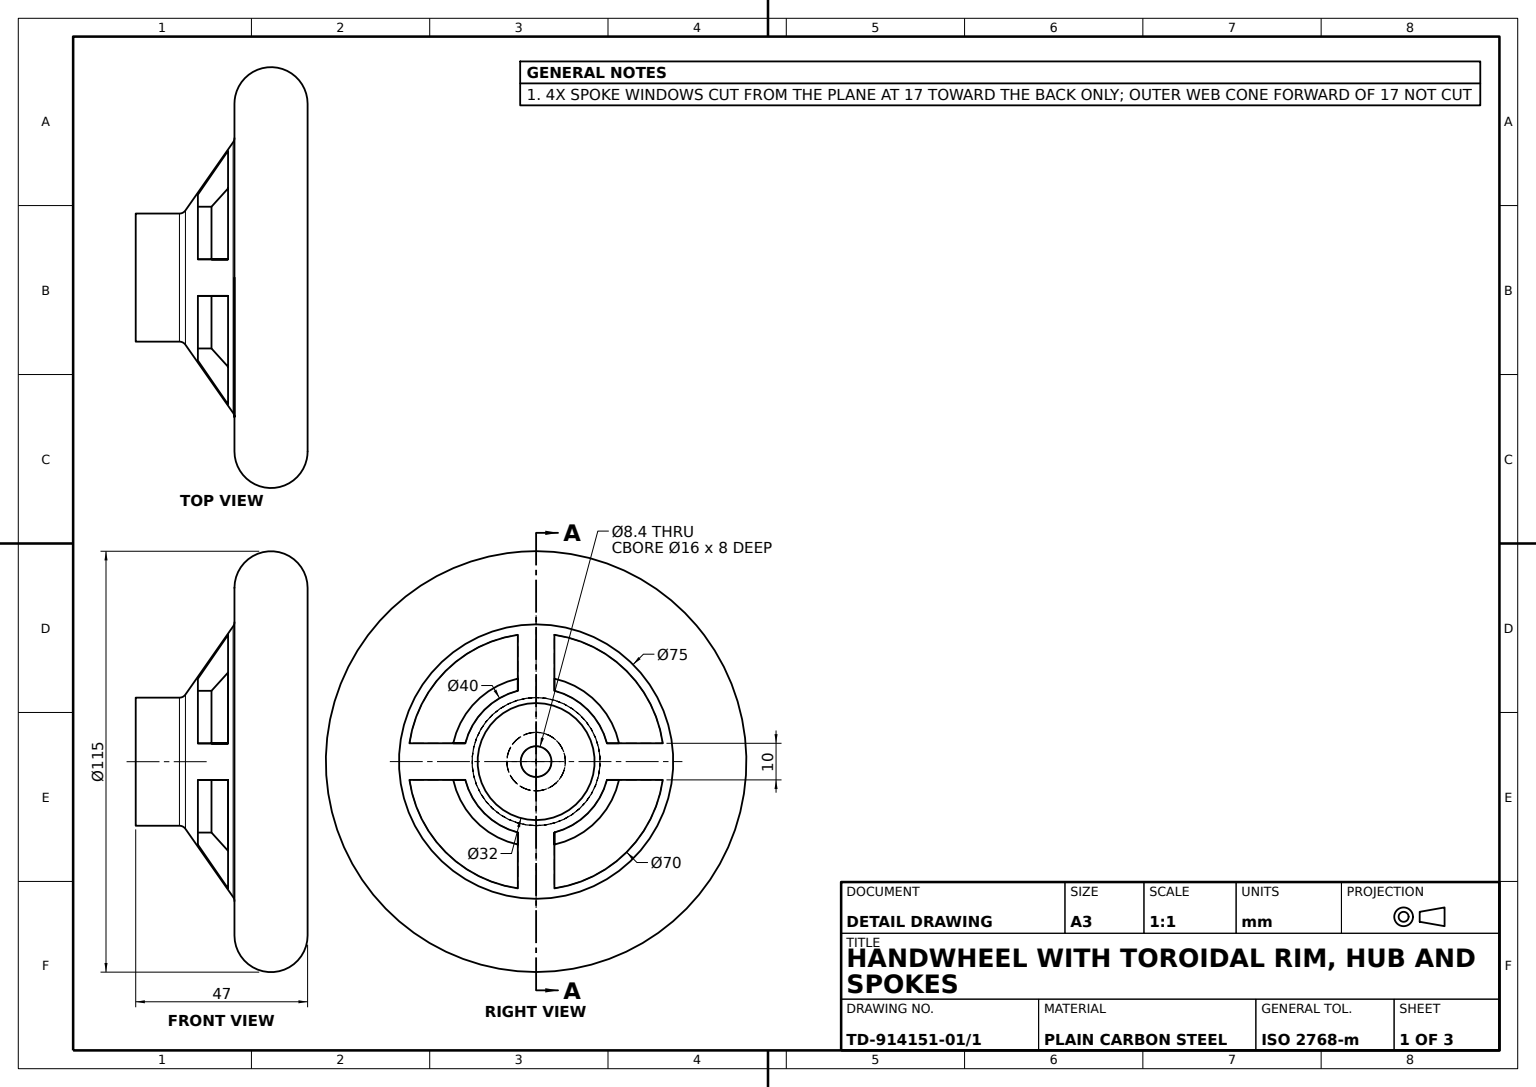
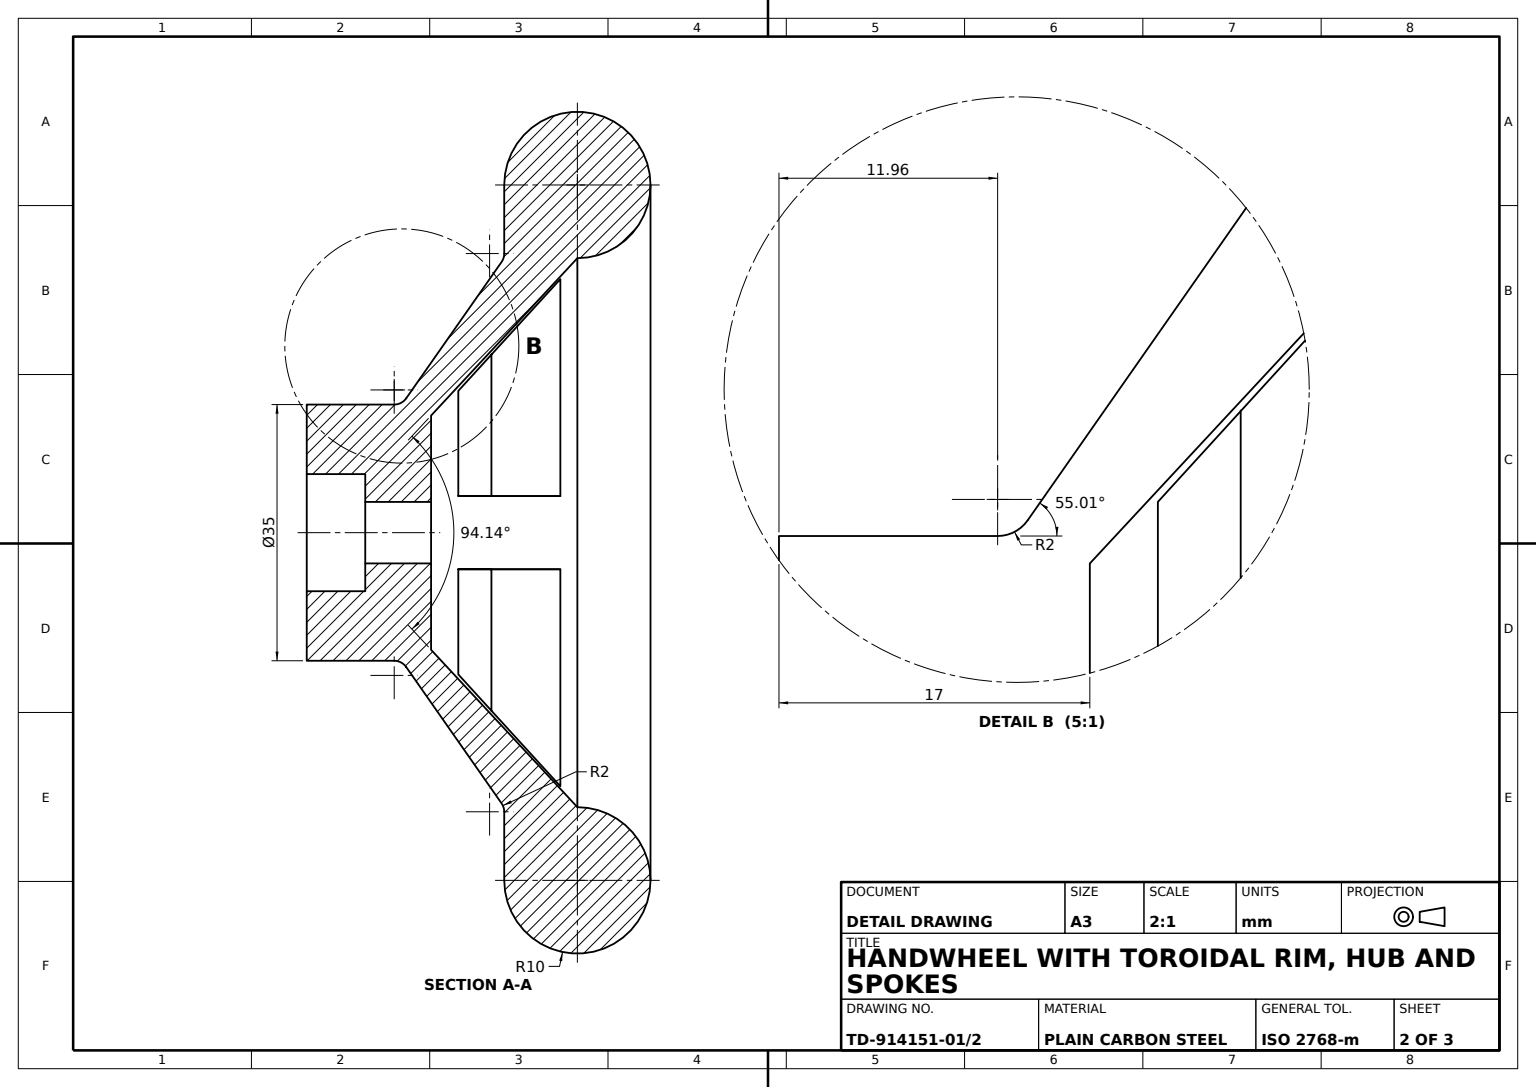
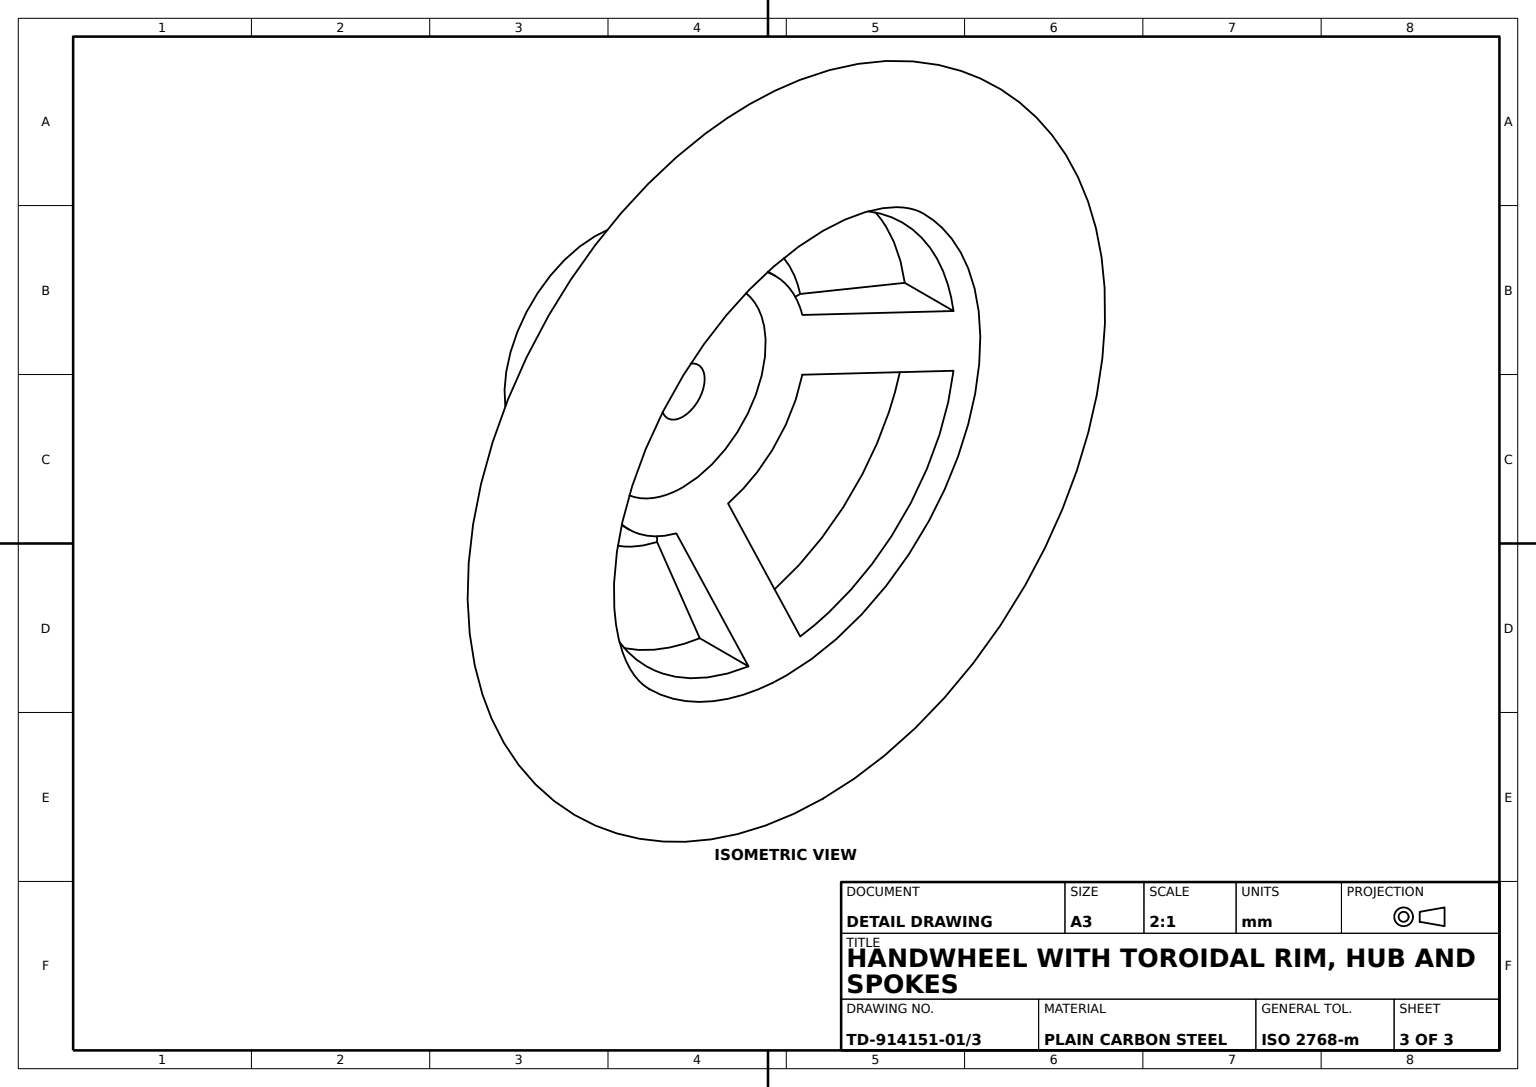
SolidWorks part; units mm, degrees
material "Plain Carbon Steel"
ref_plane "Front Plane" through (0, 0, 0) normal (0, 0, 1) x (1, 0, 0)
ref_plane "Top Plane" through (0, 0, 0) normal (0, 1, 0) x (1, 0, 0)
ref_plane "Right Plane" through (0, 0, 0) normal (1, 0, 0) x (0, 0, -1)
sketch "Handwheel Profile Sketch" plane through (0, 0, 0) normal (0, 0, 1) x (1, 0, 0)
  line L0 (0, 48.5307) -> (0, -37) construction
  line L1 (-8, -37) -> (-17.5, -37)
  line L2 (-17.5, -37) -> (-17.5, -25.0413)
  line L3 (-4.2, -20) -> (-4.2, -29)
  line L4 (-47.5, -10) -> (-38.1304, -10)
  line L5 (-36.9835, -10.3615) -> (-18.3531, -23.4028)
  line L6 (-4.2, -20) -> (-16, -20)
  line L7 (-37.5, 0) -> (-16, -20)
  line L11 (-4.2, -29) -> (-8, -29)
  line L12 (-8, -37) -> (-8, -29)
  arc A4 (-37.5, 0) -> (-47.5, -10) centre (-47.5, 0) ccw
  arc A5 (-38.1304, -10) -> (-36.9835, -10.3615) centre (-38.1304, -12) cw
  arc A6 (-17.5, -25.0413) -> (-18.3531, -23.4028) centre (-19.5, -25.0413) ccw
  point P9 (-47.5, 10)
  point P11 (0, -20)
  point P12 (-17.5, -20)
  point P16 (-37.5, -10)
  point P19 (-17.5, -24)
  point P20 (0, -37.605)
  dimension "D1" = 20
  dimension "D2" = 47.5
  dimension "D3" = 17.5
  dimension "D7" = 2
  dimension "D4" = 13
  dimension "D5" = 10
  dimension "D6" = 37
  dimension "D8" = 8
  dimension "D9" = 8
  dimension "D10" = 4.2
  dimension "D11" = 16
  dimension "D12" = 17
  dimension "D13" = 0.605
revolve "Handwheel Body" add sketch "Handwheel Profile Sketch" angle 360 about L0
sketch "Spoke Windows Sketch" plane through (0, -20, 0) normal (0, 1, 0) x (1, 0, 0)
  line L0 (0, 37.5) -> (0, -37.5) construction
  line L1 (-5, 34.641) -> (-5, 19.3649)
  line L2 (5, 34.641) -> (5, 19.3649)
  line L3 (-37.5, 0) -> (37.5, 0) construction
  line L4 (-34.641, -5) -> (-19.3649, -5)
  line L5 (-34.641, 5) -> (-19.3649, 5)
  line L6 (-5, 5) -> (-5, -5)
  line L7 (-5, 5) -> (5, 5)
  line L8 (-5, 37.5) -> (-5, -37.5) construction
  line L9 (5, 5) -> (5, -5)
  line L10 (-37.5, 5) -> (37.5, 5) construction
  line L11 (19.3649, 5) -> (34.641, 5)
  line L12 (5, 37.5) -> (5, -37.5) construction
  line L13 (19.3649, -5) -> (34.641, -5)
  line L14 (-5, -5) -> (5, -5)
  line L15 (-37.5, -5) -> (37.5, -5) construction
  line L16 (-5, -19.3649) -> (-5, -34.641)
  line L17 (5, -19.3649) -> (5, -34.641)
  circle A0 centre (0, 0) radius 37.5 construction
  arc A1 (-34.641, -5) -> (-5, -34.641) centre (0, 0) ccw
  arc A2 (-19.3649, -5) -> (-5, -19.3649) centre (0, 0) ccw
  arc A3 (0, -20) -> (19.3649, -5) centre (0, 0) ccw
  arc A4 (5, -34.641) -> (34.641, -5) centre (0, 0) ccw
  arc A5 (19.3649, 5) -> (5, 19.3649) centre (0, 0) ccw
  arc A6 (34.641, 5) -> (5, 34.641) centre (0, 0) ccw
  arc A7 (-5, 34.641) -> (-34.641, 5) centre (0, 0) ccw
  arc A8 (-5, 19.3649) -> (-19.3649, 5) centre (0, 0) ccw
  dimension "D3" = 70
  dimension "D4" = 40
  dimension "D1" = 5
  dimension "D2" = 5
  dimension "D5" = 5
  dimension "D6" = 5
extrude "Spoke Windows 4x" cut sketch "Spoke Windows Sketch" along normal blind 20 contours L11 A6 L2 A5 | L17 A4 L13 A3 | A7 L5 A8 L1 | A1 L16 A2 L4
